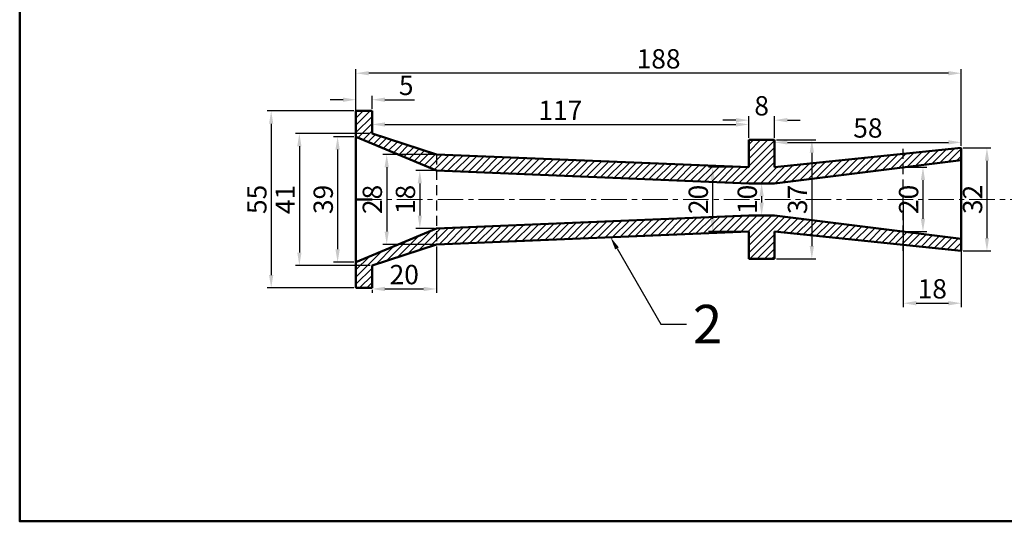
# Model space of a CAD drawing. Units: millimetres. Extents: x 39 to 520, y -165 to 464.
# Tile 1 of 4: x 39 to 345, y -165 to -9. Entities that reach past the tile are written whole.
import ezdxf
from ezdxf import colors
from ezdxf.entities.mleader import LeaderData, LeaderLine
from ezdxf.math import Vec2, Vec3

# ---------------------------------------------------------------- set-up
doc = ezdxf.new("R2010")
doc.units = ezdxf.units.MM
doc.header["$LTSCALE"] = 0.5
doc.linetypes.add('CENTER', pattern=[50.8, 31.75, -6.35, 6.35, -6.35])
doc.linetypes.add('DASHED', pattern=[19.05, 12.7, -6.35])
for name, color, linetype, lineweight in [('M-CNTR', 1, 'CENTER', 18), ('M-DIMS', 2, 'Continuous', 25), ('M-HATC', 8, 'Continuous', 18), ('M-HIDN', 6, 'DASHED', 25), ('M-OUTL', 7, 'Continuous', 50), ('M-TEXT', 3, 'Continuous', 25), ('M-TTLB', 7, 'Continuous', 50)]:
    doc.layers.add(name, color=color, linetype=linetype, lineweight=lineweight)
doc.styles.get("Standard").update_dxf_attribs({"font": 'arial.ttf'})
doc.dimstyles.new('ISO-25', dxfattribs={"dimtxt": 6, "dimasz": 4, "dimexe": 1.25, "dimexo": 0.625, "dimtad": 1, "dimtoh": 1, "dimdec": 1, "dimtxsty": 'Standard', "dimcen": 2.5, "dimadec": 0, "dimazin": 0, "dimtfac": 1, "dimtdec": 1, "dimtofl": 0, "dimtmove": 0, "dimatfit": 3, "dimfxl": 1, "dimarcsym": 0})

# ---------------------------------------------------------------- blocks, each defined once
blk = doc.blocks.new('*D31')
at = {"layer": 'Defpoints', "color": 0, "ltscale": 0.5, "transparency": 16777216}
for p in [(313.7, -65.06), (331.7, -65.06), (331.7, -97.31)]:
    blk.add_point(p, dxfattribs=at)
at = {"layer": 'M-DIMS', "color": 0, "lineweight": -2, "ltscale": 0.5, "transparency": 16777216}
for p, q in [((313.7, -65.69), (313.7, -98.56)), ((331.7, -65.69), (331.7, -98.56)), ((317.7, -97.31), (327.7, -97.31))]:
    blk.add_line(p, q, dxfattribs=at)
at = {"layer": 'M-DIMS', "color": 0, "ltscale": 0.5, "transparency": 16777216}
for points in [[(317.7, -96.64), (317.7, -97.98), (313.7, -97.31)], [(327.7, -96.64), (327.7, -97.98), (331.7, -97.31)]]:
    blk.add_solid(points, dxfattribs=at)
at = {"layer": 'M-DIMS', "color": 0, "ltscale": 0.5, "transparency": 16777216, "insert": (322.7, -93.62), "char_height": 6, "attachment_point": 5}
blk.add_mtext('18', dxfattribs=at)
blk = doc.blocks.new('*D32')
at = {"layer": 'Defpoints', "color": 0, "ltscale": 0.5, "transparency": 16777216}
for p in [(313.7, -55.06), (313.7, -75.06), (319.81, -75.06)]:
    blk.add_point(p, dxfattribs=at)
at = {"layer": 'M-DIMS', "color": 0, "lineweight": -2, "ltscale": 0.5, "transparency": 16777216}
for p, q in [((314.33, -55.06), (321.06, -55.06)), ((319.81, -59.06), (319.81, -71.06)), ((314.33, -75.06), (321.06, -75.06))]:
    blk.add_line(p, q, dxfattribs=at)
at = {"layer": 'M-DIMS', "color": 0, "ltscale": 0.5, "transparency": 16777216}
for points in [[(319.14, -59.06), (320.47, -59.06), (319.81, -55.06)], [(319.14, -71.06), (320.47, -71.06), (319.81, -75.06)]]:
    blk.add_solid(points, dxfattribs=at)
at = {"layer": 'M-DIMS', "color": 0, "ltscale": 0.5, "transparency": 16777216, "insert": (316.12, -65.06), "char_height": 6, "attachment_point": 5, "rotation": 90}
blk.add_mtext('20', dxfattribs=at)
blk = doc.blocks.new('*D33')
at = {"layer": 'Defpoints', "color": 0, "ltscale": 0.5, "transparency": 16777216}
for p in [(331.7, -49.06), (331.7, -81.06), (339.68, -81.06)]:
    blk.add_point(p, dxfattribs=at)
at = {"layer": 'M-DIMS', "color": 0, "lineweight": -2, "ltscale": 0.5, "transparency": 16777216}
for p, q in [((332.33, -49.06), (340.93, -49.06)), ((339.68, -53.06), (339.68, -77.06)), ((332.33, -81.06), (340.93, -81.06))]:
    blk.add_line(p, q, dxfattribs=at)
at = {"layer": 'M-DIMS', "color": 0, "ltscale": 0.5, "transparency": 16777216}
for points in [[(339.01, -53.06), (340.34, -53.06), (339.68, -49.06)], [(339.01, -77.06), (340.34, -77.06), (339.68, -81.06)]]:
    blk.add_solid(points, dxfattribs=at)
at = {"layer": 'M-DIMS', "color": 0, "ltscale": 0.5, "transparency": 16777216, "insert": (335.99, -65.06), "char_height": 6, "attachment_point": 5, "rotation": 90}
blk.add_mtext('32', dxfattribs=at)
blk = doc.blocks.new('*D34')
at = {"layer": 'Defpoints', "color": 0, "ltscale": 0.5, "transparency": 16777216}
for p in [(273.7, -40.43), (265.7, -46.56), (273.7, -46.56)]:
    blk.add_point(p, dxfattribs=at)
at = {"layer": 'M-DIMS', "color": 0, "lineweight": -2, "ltscale": 0.5, "transparency": 16777216}
for p, q in [((265.7, -45.94), (265.7, -39.18)), ((273.7, -45.94), (273.7, -39.18)), ((261.7, -40.43), (257.7, -40.43)), ((277.7, -40.43), (281.7, -40.43))]:
    blk.add_line(p, q, dxfattribs=at)
at = {"layer": 'M-DIMS', "color": 0, "ltscale": 0.5, "transparency": 16777216}
for points in [[(261.7, -39.76), (261.7, -41.09), (265.7, -40.43)], [(277.7, -39.76), (277.7, -41.09), (273.7, -40.43)]]:
    blk.add_solid(points, dxfattribs=at)
at = {"layer": 'M-DIMS', "color": 0, "ltscale": 0.5, "transparency": 16777216, "insert": (269.7, -36.74), "char_height": 6, "attachment_point": 5}
blk.add_mtext('8', dxfattribs=at)
blk = doc.blocks.new('*D35')
at = {"layer": 'Defpoints', "color": 0, "ltscale": 0.5, "transparency": 16777216}
for p in [(143.7, -25.84), (143.7, -49.06), (331.7, -49.06)]:
    blk.add_point(p, dxfattribs=at)
at = {"layer": 'M-DIMS', "color": 0, "lineweight": -2, "ltscale": 0.5, "transparency": 16777216}
for p, q in [((143.7, -48.44), (143.7, -24.59)), ((327.7, -25.84), (147.7, -25.84)), ((331.7, -48.44), (331.7, -24.59))]:
    blk.add_line(p, q, dxfattribs=at)
at = {"layer": 'M-DIMS', "color": 0, "ltscale": 0.5, "transparency": 16777216}
for points in [[(147.7, -25.17), (147.7, -26.51), (143.7, -25.84)], [(327.7, -25.17), (327.7, -26.51), (331.7, -25.84)]]:
    blk.add_solid(points, dxfattribs=at)
at = {"layer": 'M-DIMS', "color": 0, "ltscale": 0.5, "transparency": 16777216, "insert": (237.7, -22.15), "char_height": 6, "attachment_point": 5}
blk.add_mtext('188', dxfattribs=at)
blk = doc.blocks.new('*D36')
at = {"layer": 'Defpoints', "color": 0, "ltscale": 0.5, "transparency": 16777216}
for p in [(148.7, -34.08), (143.7, -37.56), (148.7, -37.56)]:
    blk.add_point(p, dxfattribs=at)
at = {"layer": 'M-DIMS', "color": 0, "lineweight": -2, "ltscale": 0.5, "transparency": 16777216}
for p, q in [((143.7, -36.94), (143.7, -32.83)), ((148.7, -36.94), (148.7, -32.83)), ((139.7, -34.08), (135.7, -34.08)), ((152.7, -34.08), (161.93, -34.08))]:
    blk.add_line(p, q, dxfattribs=at)
at = {"layer": 'M-DIMS', "color": 0, "ltscale": 0.5, "transparency": 16777216}
for points in [[(139.7, -33.41), (139.7, -34.74), (143.7, -34.08)], [(152.7, -33.41), (152.7, -34.74), (148.7, -34.08)]]:
    blk.add_solid(points, dxfattribs=at)
at = {"layer": 'M-DIMS', "color": 0, "ltscale": 0.5, "transparency": 16777216, "insert": (159.32, -30.4), "char_height": 6, "attachment_point": 5}
blk.add_mtext('5', dxfattribs=at)
blk = doc.blocks.new('*D37')
at = {"layer": 'Defpoints', "color": 0, "ltscale": 0.5, "transparency": 16777216}
for p in [(143.7, -37.56), (117.38, -92.56), (143.7, -92.56)]:
    blk.add_point(p, dxfattribs=at)
at = {"layer": 'M-DIMS', "color": 0, "lineweight": -2, "ltscale": 0.5, "transparency": 16777216}
for p, q in [((143.08, -37.56), (116.13, -37.56)), ((117.38, -41.56), (117.38, -88.56)), ((143.08, -92.56), (116.13, -92.56))]:
    blk.add_line(p, q, dxfattribs=at)
at = {"layer": 'M-DIMS', "color": 0, "ltscale": 0.5, "transparency": 16777216}
for points in [[(116.71, -41.56), (118.04, -41.56), (117.38, -37.56)], [(116.71, -88.56), (118.04, -88.56), (117.38, -92.56)]]:
    blk.add_solid(points, dxfattribs=at)
at = {"layer": 'M-DIMS', "color": 0, "ltscale": 0.5, "transparency": 16777216, "insert": (113.7, -65.06), "char_height": 6, "attachment_point": 5, "rotation": 90}
blk.add_mtext('55', dxfattribs=at)
blk = doc.blocks.new('*D38')
at = {"layer": 'Defpoints', "color": 0, "ltscale": 0.5, "transparency": 16777216}
for p in [(143.7, -45.56), (138.01, -84.56), (143.7, -84.56)]:
    blk.add_point(p, dxfattribs=at)
at = {"layer": 'M-DIMS', "color": 0, "lineweight": -2, "ltscale": 0.5, "transparency": 16777216}
for p, q in [((143.08, -45.56), (136.76, -45.56)), ((138.01, -49.56), (138.01, -80.56)), ((143.08, -84.56), (136.76, -84.56))]:
    blk.add_line(p, q, dxfattribs=at)
at = {"layer": 'M-DIMS', "color": 0, "ltscale": 0.5, "transparency": 16777216}
for points in [[(137.34, -49.56), (138.68, -49.56), (138.01, -45.56)], [(137.34, -80.56), (138.68, -80.56), (138.01, -84.56)]]:
    blk.add_solid(points, dxfattribs=at)
at = {"layer": 'M-DIMS', "color": 0, "ltscale": 0.5, "transparency": 16777216, "insert": (134.32, -65.06), "char_height": 6, "attachment_point": 5, "rotation": 90}
blk.add_mtext('39', dxfattribs=at)
blk = doc.blocks.new('*D39')
at = {"layer": 'Defpoints', "color": 0, "ltscale": 0.5, "transparency": 16777216}
for p in [(148.7, -44.56), (126.13, -85.56), (148.7, -85.56)]:
    blk.add_point(p, dxfattribs=at)
at = {"layer": 'M-DIMS', "color": 0, "lineweight": -2, "ltscale": 0.5, "transparency": 16777216}
for p, q in [((148.08, -44.56), (124.88, -44.56)), ((126.13, -48.56), (126.13, -81.56)), ((148.08, -85.56), (124.88, -85.56))]:
    blk.add_line(p, q, dxfattribs=at)
at = {"layer": 'M-DIMS', "color": 0, "ltscale": 0.5, "transparency": 16777216}
for points in [[(125.47, -48.56), (126.8, -48.56), (126.13, -44.56)], [(125.47, -81.56), (126.8, -81.56), (126.13, -85.56)]]:
    blk.add_solid(points, dxfattribs=at)
at = {"layer": 'M-DIMS', "color": 0, "ltscale": 0.5, "transparency": 16777216, "insert": (122.5, -65.06), "char_height": 6, "attachment_point": 5, "rotation": 90}
blk.add_mtext('41', dxfattribs=at)
blk = doc.blocks.new('*D40')
at = {"layer": 'Defpoints', "color": 0, "ltscale": 0.5, "transparency": 16777216}
for p in [(168.91, -51.07), (153.26, -79.06), (168.7, -79.06)]:
    blk.add_point(p, dxfattribs=at)
at = {"layer": 'M-DIMS', "color": 0, "lineweight": -2, "ltscale": 0.5, "transparency": 16777216}
for p, q in [((168.28, -51.07), (152.01, -51.07)), ((153.26, -55.07), (153.26, -75.06)), ((168.08, -79.06), (152.01, -79.06))]:
    blk.add_line(p, q, dxfattribs=at)
at = {"layer": 'M-DIMS', "color": 0, "ltscale": 0.5, "transparency": 16777216}
for points in [[(152.6, -55.07), (153.93, -55.07), (153.26, -51.07)], [(152.6, -75.06), (153.93, -75.06), (153.26, -79.06)]]:
    blk.add_solid(points, dxfattribs=at)
at = {"layer": 'M-DIMS', "color": 0, "ltscale": 0.5, "transparency": 16777216, "insert": (149.57, -65.06), "char_height": 6, "attachment_point": 5, "rotation": 90}
blk.add_mtext('28', dxfattribs=at)
blk = doc.blocks.new('*D41')
at = {"layer": 'Defpoints', "color": 0, "ltscale": 0.5, "transparency": 16777216}
for p in [(168.7, -56.06), (163.54, -74.06), (168.7, -74.06)]:
    blk.add_point(p, dxfattribs=at)
at = {"layer": 'M-DIMS', "color": 0, "lineweight": -2, "ltscale": 0.5, "transparency": 16777216}
for p, q in [((168.08, -56.06), (162.29, -56.06)), ((163.54, -60.06), (163.54, -70.06)), ((168.08, -74.06), (162.29, -74.06))]:
    blk.add_line(p, q, dxfattribs=at)
at = {"layer": 'M-DIMS', "color": 0, "ltscale": 0.5, "transparency": 16777216}
for points in [[(162.88, -60.06), (164.21, -60.06), (163.54, -56.06)], [(162.88, -70.06), (164.21, -70.06), (163.54, -74.06)]]:
    blk.add_solid(points, dxfattribs=at)
at = {"layer": 'M-DIMS', "color": 0, "ltscale": 0.5, "transparency": 16777216, "insert": (159.85, -65.06), "char_height": 6, "attachment_point": 5, "rotation": 90}
blk.add_mtext('18', dxfattribs=at)
blk = doc.blocks.new('*D42')
at = {"layer": 'Defpoints', "color": 0, "ltscale": 0.5, "transparency": 16777216}
for p in [(168.7, -79.06), (148.7, -92.56), (168.7, -92.88)]:
    blk.add_point(p, dxfattribs=at)
at = {"layer": 'M-DIMS', "color": 0, "lineweight": -2, "ltscale": 0.5, "transparency": 16777216}
for p, q in [((168.7, -79.69), (168.7, -94.13)), ((148.7, -93.19), (148.7, -94.13)), ((152.7, -92.88), (164.7, -92.88))]:
    blk.add_line(p, q, dxfattribs=at)
at = {"layer": 'M-DIMS', "color": 0, "ltscale": 0.5, "transparency": 16777216}
for points in [[(152.7, -92.21), (152.7, -93.55), (148.7, -92.88)], [(164.7, -92.21), (164.7, -93.55), (168.7, -92.88)]]:
    blk.add_solid(points, dxfattribs=at)
at = {"layer": 'M-DIMS', "color": 0, "ltscale": 0.5, "transparency": 16777216, "insert": (158.7, -89.19), "char_height": 6, "attachment_point": 5}
blk.add_mtext('20', dxfattribs=at)
blk = doc.blocks.new('*D43')
at = {"layer": 'Defpoints', "color": 0, "ltscale": 0.5, "transparency": 16777216}
for p in [(148.7, -41.06), (265.7, -41.76), (265.7, -46.56)]:
    blk.add_point(p, dxfattribs=at)
at = {"layer": 'M-DIMS', "color": 0, "lineweight": -2, "ltscale": 0.5, "transparency": 16777216}
for p, q in [((148.7, -41.69), (148.7, -43.01)), ((152.7, -41.76), (261.7, -41.76)), ((265.7, -45.94), (265.7, -40.51))]:
    blk.add_line(p, q, dxfattribs=at)
at = {"layer": 'M-DIMS', "color": 0, "ltscale": 0.5, "transparency": 16777216}
for points in [[(152.7, -41.1), (152.7, -42.43), (148.7, -41.76)], [(261.7, -41.1), (261.7, -42.43), (265.7, -41.76)]]:
    blk.add_solid(points, dxfattribs=at)
at = {"layer": 'M-DIMS', "color": 0, "ltscale": 0.5, "transparency": 16777216, "insert": (207.2, -38.13), "char_height": 6, "attachment_point": 5}
blk.add_mtext('117', dxfattribs=at)
blk = doc.blocks.new('*D44')
at = {"layer": 'Defpoints', "color": 0, "ltscale": 0.5, "transparency": 16777216}
for p in [(273.7, -46.56), (331.7, -47.33), (331.7, -49.06)]:
    blk.add_point(p, dxfattribs=at)
at = {"layer": 'M-DIMS', "color": 0, "lineweight": -2, "ltscale": 0.5, "transparency": 16777216}
for p, q in [((273.7, -47.19), (273.7, -48.58)), ((277.7, -47.33), (327.7, -47.33)), ((331.7, -48.44), (331.7, -46.08))]:
    blk.add_line(p, q, dxfattribs=at)
at = {"layer": 'M-DIMS', "color": 0, "ltscale": 0.5, "transparency": 16777216}
for points in [[(277.7, -46.66), (277.7, -47.99), (273.7, -47.33)], [(327.7, -46.66), (327.7, -47.99), (331.7, -47.33)]]:
    blk.add_solid(points, dxfattribs=at)
at = {"layer": 'M-DIMS', "color": 0, "ltscale": 0.5, "transparency": 16777216, "insert": (302.7, -43.64), "char_height": 6, "attachment_point": 5}
blk.add_mtext('58', dxfattribs=at)
blk = doc.blocks.new('*D45')
at = {"layer": 'Defpoints', "color": 0, "ltscale": 0.5, "transparency": 16777216}
for p in [(265.7, -55.06), (254.49, -75.06), (265.7, -75.06)]:
    blk.add_point(p, dxfattribs=at)
at = {"layer": 'M-DIMS', "color": 0, "lineweight": -2, "ltscale": 0.5, "transparency": 16777216}
for p, q in [((265.08, -55.06), (253.24, -55.06)), ((254.49, -59.06), (254.49, -71.06)), ((265.08, -75.06), (253.24, -75.06))]:
    blk.add_line(p, q, dxfattribs=at)
at = {"layer": 'M-DIMS', "color": 0, "ltscale": 0.5, "transparency": 16777216}
for points in [[(253.82, -59.06), (255.16, -59.06), (254.49, -55.06)], [(253.82, -71.06), (255.16, -71.06), (254.49, -75.06)]]:
    blk.add_solid(points, dxfattribs=at)
at = {"layer": 'M-DIMS', "color": 0, "ltscale": 0.5, "transparency": 16777216, "insert": (250.8, -65.06), "char_height": 6, "attachment_point": 5, "rotation": 90}
blk.add_mtext('20', dxfattribs=at)
blk = doc.blocks.new('*D46')
at = {"layer": 'Defpoints', "color": 0, "ltscale": 0.5, "transparency": 16777216}
for p in [(269.7, -60.06), (269.7, -70.06), (269.7, -70.06)]:
    blk.add_point(p, dxfattribs=at)
at = {"layer": 'M-DIMS', "color": 0, "lineweight": -2, "ltscale": 0.5, "transparency": 16777216}
for p, q in [((270.33, -60.06), (270.95, -60.06)), ((269.7, -64.06), (269.7, -66.06)), ((270.33, -70.06), (270.95, -70.06))]:
    blk.add_line(p, q, dxfattribs=at)
at = {"layer": 'M-DIMS', "color": 0, "ltscale": 0.5, "transparency": 16777216}
for points in [[(269.04, -64.06), (270.37, -64.06), (269.7, -60.06)], [(269.04, -66.06), (270.37, -66.06), (269.7, -70.06)]]:
    blk.add_solid(points, dxfattribs=at)
at = {"layer": 'M-DIMS', "color": 0, "ltscale": 0.5, "transparency": 16777216, "insert": (266.01, -65.06), "char_height": 6, "attachment_point": 5, "rotation": 90}
blk.add_mtext('10', dxfattribs=at)
blk = doc.blocks.new('*D47')
at = {"layer": 'Defpoints', "color": 0, "ltscale": 0.5, "transparency": 16777216}
for p in [(273.7, -46.56), (273.7, -83.56), (285.3, -83.56)]:
    blk.add_point(p, dxfattribs=at)
at = {"layer": 'M-DIMS', "color": 0, "lineweight": -2, "ltscale": 0.5, "transparency": 16777216}
for p, q in [((274.33, -46.56), (286.55, -46.56)), ((285.3, -50.56), (285.3, -79.56)), ((274.33, -83.56), (286.55, -83.56))]:
    blk.add_line(p, q, dxfattribs=at)
at = {"layer": 'M-DIMS', "color": 0, "ltscale": 0.5, "transparency": 16777216}
for points in [[(284.63, -50.56), (285.97, -50.56), (285.3, -46.56)], [(284.63, -79.56), (285.97, -79.56), (285.3, -83.56)]]:
    blk.add_solid(points, dxfattribs=at)
at = {"layer": 'M-DIMS', "color": 0, "ltscale": 0.5, "transparency": 16777216, "insert": (281.61, -65.06), "char_height": 6, "attachment_point": 5, "rotation": 90}
blk.add_mtext('37', dxfattribs=at)

msp = doc.modelspace()

# ---------------------------------------------------------------- hatches: boundary and pattern name
at = {"layer": 'M-HATC', "ltscale": 0.5}
h = msp.add_hatch(dxfattribs=at)
h.set_pattern_fill('ANSI31', color=256, scale=0.5)
h.set_pattern_definition([(45, (-145.7227, 1323.1625), (-1.122532, 1.122532), [])])
h.paths.add_polyline_path([(313.7018, -55.0616), (313.7018, -50.9237), (273.7018, -55.0616), (273.7018, -46.5616), (265.7018, -46.5616), (265.7018, -55.0616), (168.7018, -51.0616), (168.7018, -56.0616), (265.7018, -60.0616), (273.7018, -60.0616)])
h.paths.add_polyline_path([(168.7018, -79.0616), (168.7018, -74.0616), (143.7018, -84.5616), (143.7018, -92.5616), (148.7018, -92.5616), (148.7018, -85.5616)])
h.paths.add_polyline_path([(148.7018, -44.5616), (148.7018, -37.5616), (143.7018, -37.5616), (143.7018, -45.5616), (168.7018, -56.0616), (168.7018, -51.0616)])
h.paths.add_polyline_path([(265.7018, -75.0616), (265.7018, -83.5616), (273.7018, -83.5616), (273.7018, -75.0616), (313.7018, -79.1995), (313.7018, -75.0616), (273.7018, -70.0616), (265.7018, -70.0616), (168.7018, -74.0616), (168.7018, -79.0616)])
h.paths.add_polyline_path([(331.7018, -49.0616), (313.7018, -50.9237), (313.7018, -55.0616), (331.7018, -52.8116)])
h.paths.add_polyline_path([(313.7018, -75.0616), (313.7018, -79.1995), (331.7018, -81.0616), (331.7018, -77.3116)])

# ---------------------------------------------------------------- linework, layer by layer
at = {"layer": 'M-CNTR', "ltscale": 0.5}
msp.add_line((143.7018, -65.0616), (412.7093, -65.0616), dxfattribs=at)
at = {"layer": 'M-HIDN', "ltscale": 0.5}
for p, q in [((168.7018, -51.0616), (168.7018, -79.0616)), ((313.7018, -81.0616), (313.7018, -49.0616))]:
    msp.add_line(p, q, dxfattribs=at)
at = {"layer": 'M-OUTL', "ltscale": 0.5}
for p, q in [((143.7018, -37.5616), (143.7018, -92.5616)), ((148.7018, -37.5616), (143.7018, -37.5616)), ((148.7018, -44.5616), (148.7018, -37.5616)), ((168.7018, -56.0616), (143.7018, -45.5616)), ((148.7018, -44.5616), (168.7018, -51.0616)), ((273.7018, -46.5616), (265.7018, -46.5616)), ((273.7018, -46.5616), (265.7018, -46.5616)), ((265.7018, -46.5616), (265.7018, -55.0616)), ((273.7018, -55.0616), (273.7018, -46.5616)), ((168.7018, -51.0616), (265.7018, -55.0616)), ((273.7018, -55.0616), (331.7018, -49.0616)), ((331.7018, -81.0616), (331.7018, -49.0616)), ((273.7018, -60.0616), (331.7018, -52.8116)), ((168.7018, -56.0616), (265.7018, -60.0616)), ((265.7018, -60.0616), (273.7018, -60.0616)), ((143.7018, -65.0616), (148.7018, -65.0616)), ((168.7018, -74.0616), (265.7018, -70.0616)), ((265.7018, -70.0616), (273.7018, -70.0616)), ((273.7018, -70.0616), (331.7018, -77.3116)), ((168.7018, -74.0616), (143.7018, -84.5616)), ((168.7018, -79.0616), (265.7018, -75.0616)), ((265.7018, -75.0616), (265.7018, -83.5616)), ((273.7018, -83.5616), (273.7018, -75.0616)), ((331.7018, -81.0616), (273.7018, -75.0616)), ((148.7018, -85.5616), (168.7018, -79.0616)), ((148.7018, -92.5616), (148.7018, -85.5616)), ((273.7018, -83.5616), (265.7018, -83.5616)), ((143.7018, -92.5616), (148.7018, -92.5616))]:
    msp.add_line(p, q, dxfattribs=at)
at = {"layer": 'M-TTLB', "ltscale": 0.5}
msp.add_lwpolyline([(39.27, 463.9335), (519.8288, 463.9335), (519.8288, -165.0878), (39.27, -165.0878)], close=True, dxfattribs=at)

# ---------------------------------------------------------------- dimensions: what is measured, and where the dimension line sits
at = {"layer": 'M-DIMS', "ltscale": 0.5}
for base, p1, p2, picture, middle in [((143.7018, -25.8402), (331.7018, -49.0616), (143.7018, -49.0616), '*D35', (237.7018, -22.1518)), ((148.7018, -34.0767), (143.7018, -37.5616), (148.7018, -37.5616), '*D36', (159.3159, -30.4005)), ((273.7018, -40.4267), (265.7018, -46.5616), (273.7018, -46.5616), '*D34', (269.7018, -36.7383)), ((265.7018, -41.7624), (148.7018, -41.0616), (265.7018, -46.5616), '*D43', (207.2018, -38.1251)), ((331.7018, -47.3281), (273.7018, -46.5616), (331.7018, -49.0616), '*D44', (302.7018, -43.6397)), ((331.7018, -97.3092), (313.7018, -65.0616), (331.7018, -65.0616), '*D31', (322.7018, -93.6207)), ((168.7018, -92.8784), (148.7018, -92.5616), (168.7018, -79.0616), '*D42', (158.7018, -89.1899))]:
    dim = msp.add_linear_dim(base=base, p1=p1, p2=p2, dimstyle='ISO-25', override={"dimclrd": 0, "dimclre": 0, "dimclrt": 0}, dxfattribs=at)
    dim.commit()
    dim.dimension.update_dxf_attribs({"geometry": picture, "text_midpoint": middle})
for base, p1, p2, picture, middle in [((117.3781, -92.5616), (143.7018, -37.5616), (143.7018, -92.5616), '*D37', (117.3781, -65.0616)), ((126.1339, -85.5616), (148.7018, -44.5616), (148.7018, -85.5616), '*D39', (126.1339, -65.0616)), ((138.0107, -84.5616), (143.7018, -45.5616), (143.7018, -84.5616), '*D38', (138.0107, -65.0616)), ((153.2622, -79.0616), (168.9076, -51.0701), (168.7018, -79.0616), '*D40', (153.2622, -65.0616))]:
    dim = msp.add_linear_dim(base=base, p1=p1, p2=p2, angle=90, dimstyle='ISO-25', override={"dimclrd": 0, "dimclre": 0, "dimclrt": 0}, dxfattribs=at)
    dim.commit()
    dim.dimension.update_dxf_attribs({"geometry": picture, "text_midpoint": middle, "dimtype": 160})
for base, p1, p2, picture, middle in [((285.3012, -83.5616), (273.7018, -46.5616), (273.7018, -83.5616), '*D47', (281.6107, -65.0616)), ((339.676, -81.0616), (331.7018, -49.0616), (331.7018, -81.0616), '*D33', (335.9855, -65.0616)), ((163.5429, -74.0616), (168.7018, -56.0616), (168.7018, -74.0616), '*D41', (159.8545, -65.0616)), ((254.4892, -75.0616), (265.7018, -55.0616), (265.7018, -75.0616), '*D45', (250.8007, -65.0616)), ((319.8077, -75.0616), (313.7018, -55.0616), (313.7018, -75.0616), '*D32', (316.1193, -65.0616)), ((269.7018, -70.0616), (269.7018, -60.0616), (269.7018, -70.0616), '*D46', (266.0133, -65.0616))]:
    dim = msp.add_linear_dim(base=base, p1=p1, p2=p2, angle=90, dimstyle='ISO-25', override={"dimclrd": 0, "dimclre": 0, "dimclrt": 0}, dxfattribs=at)
    dim.commit()
    dim.dimension.update_dxf_attribs({"geometry": picture, "text_midpoint": middle})

# ---------------------------------------------------------------- leaders
at = {"layer": 'M-TEXT', "ltscale": 0.5}
ml = msp.add_multileader_mtext('Standard', dxfattribs=at)
ml.set_content('2', color=256)
ml.set_leader_properties()
ml.build(insert=Vec2(0, 0))
ctx = ml.context
ctx.base_point, ctx.char_height, ctx.plane_origin = Vec3(246.3678, -103.8188), 12, Vec3(222.7866, -76.8313)
notes = []
notes.append((ctx, [(0, (1, 1, 0), (238.3678, -103.8188), (1, 0), 8, [(0, [(222.7866, -76.8313)], 0, [])])]))
ctx.mtext.insert, ctx.mtext.flow_direction = Vec3(248.3678, -97.8188), 5
for ctx, leaders in notes:
    for number, flags, end, landing, length, lines in leaders:
        leader = LeaderData()
        leader.index, (leader.has_last_leader_line, leader.has_dogleg_vector, leader.attachment_direction) = number, flags
        leader.last_leader_point, leader.dogleg_vector, leader.dogleg_length = Vec3(end), Vec3(landing), length
        for number, points, colour, breaks in lines:
            line = LeaderLine()
            line.index, line.vertices, line.color, line.breaks = number, Vec3.list(points), colors.encode_raw_color(colour), breaks
            leader.lines.append(line)
        ctx.leaders.append(leader)

doc.saveas('drawing.dxf')
